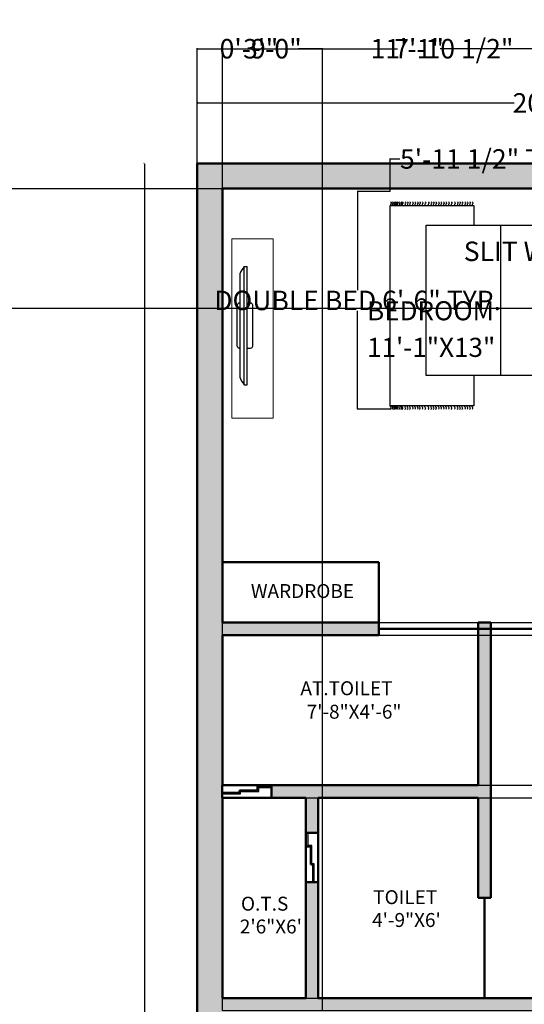
# Model space of a CAD drawing. Units: inches. Extents: x 48 to 822, y -191 to 651.
# Tile 11 of 13: x 445 to 626, y 297 to 651. Entities that reach past the tile are written whole.
import ezdxf

# ---------------------------------------------------------------- set-up
doc = ezdxf.new("R2010")
doc.units = ezdxf.units.IN
doc.header["$MEASUREMENT"] = 0
doc.layers.get('0').update_dxf_attribs({"color": 254})
for name, color, linetype, lineweight in [('A-ANNO-DIMS', 2, 'Continuous', 18), ('A-AREA-IDEN', 7, 'Continuous', 25), ('A-FURN', 8, 'Continuous', 18), ('A-GLAZ', 4, 'Continuous', 25), ('A-WALL', 7, 'Continuous', 50), ('A-WALL-PATT', 8, 'Continuous', 13)]:
    doc.layers.add(name, color=color, linetype=linetype, lineweight=lineweight)
doc.layers.add('furniture', color=250, linetype='Continuous')
doc.styles.get("Standard").update_dxf_attribs({"font": 'arial.ttf'})
doc.dimstyles.get("Standard").update_dxf_attribs({"dimtxt": 7, "dimasz": 0.18, "dimexe": 0.18, "dimexo": 0.0625, "dimgap": 0.09, "dimtad": 0, "dimtih": 1, "dimtoh": 1, "dimzin": 0, "dimdsep": 46, "dimlunit": 3, "dimtxsty": 'Standard', "dimcen": 0.09, "dimadec": 0, "dimazin": 0, "dimtfac": 1, "dimtofl": 0, "dimtmove": 0, "dimatfit": 3, "dimfxl": 1, "dimtolj": 1, "dimtzin": 0, "dimarcsym": 0})

# ---------------------------------------------------------------- blocks, each defined once
blk = doc.blocks.new('CARPET')
at = {"layer": 'furniture'}
for p, q in [((-51.53, -98.11), (-51.53, -55.12)), ((-51.53, -55.12), (-41.27, -55.12)), ((36, -55.12), (51.55, -55.12)), ((51.55, -55.12), (51.55, -98.11)), ((51.55, -98.11), (-51.53, -98.11))]:
    blk.add_line(p, q, dxfattribs=at)
for points, knots in [([(-53.37, -55.99), (-53.22, -55.8), (-52.9, -55.41), (-52.34, -55.8), (-51.89, -56.08), (-51.65, -55.91), (-51.53, -55.83)], [0, 0, 0, 0, 0.653278, 1.290138, 1.740457, 2.114451, 2.114451, 2.114451, 2.114451]), ([(53.37, -55.99), (53.22, -55.8), (52.9, -55.41), (52.34, -55.8), (51.89, -56.08), (51.65, -55.91), (51.53, -55.83)], [0, 0, 0, 0, 0.653278, 1.290138, 1.740457, 2.114451, 2.114451, 2.114451, 2.114451]), ([(-53.37, -57.26), (-53.22, -57.07), (-52.9, -56.67), (-52.34, -57.07), (-51.89, -57.35), (-51.65, -57.17), (-51.53, -57.1)], [0, 0, 0, 0, 0.653278, 1.290138, 1.740457, 2.114451, 2.114451, 2.114451, 2.114451]), ([(-53.37, -58.59), (-53.22, -58.4), (-52.9, -58.01), (-52.34, -58.4), (-51.89, -58.68), (-51.65, -58.5), (-51.53, -58.43)], [0, 0, 0, 0, 0.653278, 1.290138, 1.740457, 2.114451, 2.114451, 2.114451, 2.114451]), ([(-53.37, -59.78), (-53.22, -59.58), (-52.9, -59.19), (-52.34, -59.58), (-51.89, -59.86), (-51.65, -59.69), (-51.53, -59.61)], [0, 0, 0, 0, 0.653278, 1.290138, 1.740457, 2.114451, 2.114451, 2.114451, 2.114451]), ([(-53.37, -61.22), (-53.22, -61.02), (-52.9, -60.63), (-52.34, -61.02), (-51.89, -61.3), (-51.65, -61.13), (-51.53, -61.05)], [0, 0, 0, 0, 0.653278, 1.290138, 1.740457, 2.114451, 2.114451, 2.114451, 2.114451]), ([(53.37, -57.26), (53.22, -57.07), (52.9, -56.67), (52.34, -57.07), (51.89, -57.35), (51.65, -57.17), (51.53, -57.1)], [0, 0, 0, 0, 0.653278, 1.290138, 1.740457, 2.114451, 2.114451, 2.114451, 2.114451]), ([(53.37, -58.59), (53.22, -58.4), (52.9, -58.01), (52.34, -58.4), (51.89, -58.68), (51.65, -58.5), (51.53, -58.43)], [0, 0, 0, 0, 0.653278, 1.290138, 1.740457, 2.114451, 2.114451, 2.114451, 2.114451]), ([(53.37, -59.78), (53.22, -59.58), (52.9, -59.19), (52.34, -59.58), (51.89, -59.86), (51.65, -59.69), (51.53, -59.61)], [0, 0, 0, 0, 0.653278, 1.290138, 1.740457, 2.114451, 2.114451, 2.114451, 2.114451]), ([(53.37, -61.22), (53.22, -61.02), (52.9, -60.63), (52.34, -61.02), (51.89, -61.3), (51.65, -61.13), (51.53, -61.05)], [0, 0, 0, 0, 0.653278, 1.290138, 1.740457, 2.114451, 2.114451, 2.114451, 2.114451]), ([(-53.37, -62.44), (-53.22, -62.25), (-52.9, -61.86), (-52.34, -62.25), (-51.89, -62.53), (-51.65, -62.36), (-51.53, -62.28)], [0, 0, 0, 0, 0.653278, 1.290138, 1.740457, 2.114451, 2.114451, 2.114451, 2.114451]), ([(-53.37, -63.63), (-53.22, -63.43), (-52.9, -63.04), (-52.34, -63.43), (-51.89, -63.72), (-51.65, -63.54), (-51.53, -63.46)], [0, 0, 0, 0, 0.653278, 1.290138, 1.740457, 2.114451, 2.114451, 2.114451, 2.114451]), ([(-53.37, -65.07), (-53.22, -64.87), (-52.9, -64.48), (-52.34, -64.87), (-51.89, -65.15), (-51.65, -64.98), (-51.53, -64.9)], [0, 0, 0, 0, 0.653278, 1.290138, 1.740457, 2.114451, 2.114451, 2.114451, 2.114451]), ([(53.37, -62.44), (53.22, -62.25), (52.9, -61.86), (52.34, -62.25), (51.89, -62.53), (51.65, -62.36), (51.53, -62.28)], [0, 0, 0, 0, 0.653278, 1.290138, 1.740457, 2.114451, 2.114451, 2.114451, 2.114451]), ([(53.37, -63.63), (53.22, -63.43), (52.9, -63.04), (52.34, -63.43), (51.89, -63.72), (51.65, -63.54), (51.53, -63.46)], [0, 0, 0, 0, 0.653278, 1.290138, 1.740457, 2.114451, 2.114451, 2.114451, 2.114451]), ([(53.37, -65.07), (53.22, -64.87), (52.9, -64.48), (52.34, -64.87), (51.89, -65.15), (51.65, -64.98), (51.53, -64.9)], [0, 0, 0, 0, 0.653278, 1.290138, 1.740457, 2.114451, 2.114451, 2.114451, 2.114451]), ([(-53.37, -66.76), (-53.22, -66.56), (-52.9, -66.17), (-52.34, -66.56), (-51.89, -66.84), (-51.65, -66.67), (-51.53, -66.59)], [0, 0, 0, 0, 0.653278, 1.290138, 1.740457, 2.114451, 2.114451, 2.114451, 2.114451]), ([(-53.37, -68.2), (-53.22, -68), (-52.9, -67.61), (-52.34, -68), (-51.89, -68.28), (-51.65, -68.11), (-51.53, -68.03)], [0, 0, 0, 0, 0.653278, 1.290138, 1.740457, 2.114451, 2.114451, 2.114451, 2.114451]), ([(-53.37, -69.53), (-53.22, -69.33), (-52.9, -68.94), (-52.34, -69.33), (-51.89, -69.61), (-51.65, -69.44), (-51.53, -69.36)], [0, 0, 0, 0, 0.653278, 1.290138, 1.740457, 2.114451, 2.114451, 2.114451, 2.114451]), ([(-53.37, -70.79), (-53.22, -70.6), (-52.9, -70.21), (-52.34, -70.6), (-51.89, -70.88), (-51.65, -70.7), (-51.53, -70.63)], [0, 0, 0, 0, 0.653278, 1.290138, 1.740457, 2.114451, 2.114451, 2.114451, 2.114451]), ([(53.37, -66.76), (53.22, -66.56), (52.9, -66.17), (52.34, -66.56), (51.89, -66.84), (51.65, -66.67), (51.53, -66.59)], [0, 0, 0, 0, 0.653278, 1.290138, 1.740457, 2.114451, 2.114451, 2.114451, 2.114451]), ([(53.37, -68.2), (53.22, -68), (52.9, -67.61), (52.34, -68), (51.89, -68.28), (51.65, -68.11), (51.53, -68.03)], [0, 0, 0, 0, 0.653278, 1.290138, 1.740457, 2.114451, 2.114451, 2.114451, 2.114451]), ([(53.37, -69.53), (53.22, -69.33), (52.9, -68.94), (52.34, -69.33), (51.89, -69.61), (51.65, -69.44), (51.53, -69.36)], [0, 0, 0, 0, 0.653278, 1.290138, 1.740457, 2.114451, 2.114451, 2.114451, 2.114451]), ([(53.37, -70.79), (53.22, -70.6), (52.9, -70.21), (52.34, -70.6), (51.89, -70.88), (51.65, -70.7), (51.53, -70.63)], [0, 0, 0, 0, 0.653278, 1.290138, 1.740457, 2.114451, 2.114451, 2.114451, 2.114451]), ([(-53.37, -72.12), (-53.22, -71.93), (-52.9, -71.54), (-52.34, -71.93), (-51.89, -72.21), (-51.65, -72.04), (-51.53, -71.96)], [0, 0, 0, 0, 0.653278, 1.290138, 1.740457, 2.114451, 2.114451, 2.114451, 2.114451]), ([(-53.37, -73.31), (-53.22, -73.11), (-52.9, -72.72), (-52.34, -73.11), (-51.89, -73.4), (-51.65, -73.22), (-51.53, -73.14)], [0, 0, 0, 0, 0.653278, 1.290138, 1.740457, 2.114451, 2.114451, 2.114451, 2.114451]), ([(-53.37, -74.75), (-53.22, -74.55), (-52.9, -74.16), (-52.34, -74.55), (-51.89, -74.83), (-51.65, -74.66), (-51.53, -74.58)], [0, 0, 0, 0, 0.653278, 1.290138, 1.740457, 2.114451, 2.114451, 2.114451, 2.114451]), ([(-53.37, -75.98), (-53.22, -75.78), (-52.9, -75.39), (-52.34, -75.78), (-51.89, -76.06), (-51.65, -75.89), (-51.53, -75.81)], [0, 0, 0, 0, 0.653278, 1.290138, 1.740457, 2.114451, 2.114451, 2.114451, 2.114451]), ([(53.37, -72.12), (53.22, -71.93), (52.9, -71.54), (52.34, -71.93), (51.89, -72.21), (51.65, -72.04), (51.53, -71.96)], [0, 0, 0, 0, 0.653278, 1.290138, 1.740457, 2.114451, 2.114451, 2.114451, 2.114451]), ([(53.37, -73.31), (53.22, -73.11), (52.9, -72.72), (52.34, -73.11), (51.89, -73.4), (51.65, -73.22), (51.53, -73.14)], [0, 0, 0, 0, 0.653278, 1.290138, 1.740457, 2.114451, 2.114451, 2.114451, 2.114451]), ([(53.37, -74.75), (53.22, -74.55), (52.9, -74.16), (52.34, -74.55), (51.89, -74.83), (51.65, -74.66), (51.53, -74.58)], [0, 0, 0, 0, 0.653278, 1.290138, 1.740457, 2.114451, 2.114451, 2.114451, 2.114451]), ([(53.37, -75.98), (53.22, -75.78), (52.9, -75.39), (52.34, -75.78), (51.89, -76.06), (51.65, -75.89), (51.53, -75.81)], [0, 0, 0, 0, 0.653278, 1.290138, 1.740457, 2.114451, 2.114451, 2.114451, 2.114451]), ([(-53.37, -77.16), (-53.22, -76.96), (-52.9, -76.57), (-52.34, -76.96), (-51.89, -77.25), (-51.65, -77.07), (-51.53, -76.99)], [0, 0, 0, 0, 0.653278, 1.290138, 1.740457, 2.114451, 2.114451, 2.114451, 2.114451]), ([(-53.37, -78.6), (-53.22, -78.4), (-52.9, -78.01), (-52.34, -78.4), (-51.89, -78.68), (-51.65, -78.51), (-51.53, -78.43)], [0, 0, 0, 0, 0.653278, 1.290138, 1.740457, 2.114451, 2.114451, 2.114451, 2.114451]), ([(-53.37, -80.29), (-53.22, -80.09), (-52.9, -79.7), (-52.34, -80.09), (-51.89, -80.37), (-51.65, -80.2), (-51.53, -80.12)], [0, 0, 0, 0, 0.653278, 1.290138, 1.740457, 2.114451, 2.114451, 2.114451, 2.114451]), ([(53.37, -77.16), (53.22, -76.96), (52.9, -76.57), (52.34, -76.96), (51.89, -77.25), (51.65, -77.07), (51.53, -76.99)], [0, 0, 0, 0, 0.653278, 1.290138, 1.740457, 2.114451, 2.114451, 2.114451, 2.114451]), ([(53.37, -78.6), (53.22, -78.4), (52.9, -78.01), (52.34, -78.4), (51.89, -78.68), (51.65, -78.51), (51.53, -78.43)], [0, 0, 0, 0, 0.653278, 1.290138, 1.740457, 2.114451, 2.114451, 2.114451, 2.114451]), ([(53.37, -80.29), (53.22, -80.09), (52.9, -79.7), (52.34, -80.09), (51.89, -80.37), (51.65, -80.2), (51.53, -80.12)], [0, 0, 0, 0, 0.653278, 1.290138, 1.740457, 2.114451, 2.114451, 2.114451, 2.114451]), ([(-53.37, -81.73), (-53.22, -81.53), (-52.9, -81.14), (-52.34, -81.53), (-51.89, -81.81), (-51.65, -81.64), (-51.53, -81.56)], [0, 0, 0, 0, 0.653278, 1.290138, 1.740457, 2.114451, 2.114451, 2.114451, 2.114451]), ([(-53.37, -83.06), (-53.22, -82.86), (-52.9, -82.47), (-52.34, -82.86), (-51.89, -83.14), (-51.65, -82.97), (-51.53, -82.89)], [0, 0, 0, 0, 0.653278, 1.290138, 1.740457, 2.114451, 2.114451, 2.114451, 2.114451]), ([(-53.37, -84.18), (-53.22, -83.99), (-52.9, -83.6), (-52.34, -83.99), (-51.89, -84.27), (-51.65, -84.09), (-51.53, -84.02)], [0, 0, 0, 0, 0.653278, 1.290138, 1.740457, 2.114451, 2.114451, 2.114451, 2.114451]), ([(-53.37, -85.51), (-53.22, -85.32), (-52.9, -84.93), (-52.34, -85.32), (-51.89, -85.6), (-51.65, -85.42), (-51.53, -85.35)], [0, 0, 0, 0, 0.653278, 1.290138, 1.740457, 2.114451, 2.114451, 2.114451, 2.114451]), ([(53.37, -81.73), (53.22, -81.53), (52.9, -81.14), (52.34, -81.53), (51.89, -81.81), (51.65, -81.64), (51.53, -81.56)], [0, 0, 0, 0, 0.653278, 1.290138, 1.740457, 2.114451, 2.114451, 2.114451, 2.114451]), ([(53.37, -83.06), (53.22, -82.86), (52.9, -82.47), (52.34, -82.86), (51.89, -83.14), (51.65, -82.97), (51.53, -82.89)], [0, 0, 0, 0, 0.653278, 1.290138, 1.740457, 2.114451, 2.114451, 2.114451, 2.114451]), ([(53.37, -84.18), (53.22, -83.99), (52.9, -83.6), (52.34, -83.99), (51.89, -84.27), (51.65, -84.09), (51.53, -84.02)], [0, 0, 0, 0, 0.653278, 1.290138, 1.740457, 2.114451, 2.114451, 2.114451, 2.114451]), ([(53.37, -85.51), (53.22, -85.32), (52.9, -84.93), (52.34, -85.32), (51.89, -85.6), (51.65, -85.42), (51.53, -85.35)], [0, 0, 0, 0, 0.653278, 1.290138, 1.740457, 2.114451, 2.114451, 2.114451, 2.114451]), ([(-53.37, -86.7), (-53.22, -86.5), (-52.9, -86.11), (-52.34, -86.5), (-51.89, -86.78), (-51.65, -86.61), (-51.53, -86.53)], [0, 0, 0, 0, 0.653278, 1.290138, 1.740457, 2.114451, 2.114451, 2.114451, 2.114451]), ([(-53.37, -88.14), (-53.22, -87.94), (-52.9, -87.55), (-52.34, -87.94), (-51.89, -88.22), (-51.65, -88.05), (-51.53, -87.97)], [0, 0, 0, 0, 0.653278, 1.290138, 1.740457, 2.114451, 2.114451, 2.114451, 2.114451]), ([(-53.37, -89.36), (-53.22, -89.17), (-52.9, -88.78), (-52.34, -89.17), (-51.89, -89.45), (-51.65, -89.28), (-51.53, -89.2)], [0, 0, 0, 0, 0.653278, 1.290138, 1.740457, 2.114451, 2.114451, 2.114451, 2.114451]), ([(-53.37, -90.55), (-53.22, -90.35), (-52.9, -89.96), (-52.34, -90.35), (-51.89, -90.64), (-51.65, -90.46), (-51.53, -90.38)], [0, 0, 0, 0, 0.653278, 1.290138, 1.740457, 2.114451, 2.114451, 2.114451, 2.114451]), ([(53.37, -86.7), (53.22, -86.5), (52.9, -86.11), (52.34, -86.5), (51.89, -86.78), (51.65, -86.61), (51.53, -86.53)], [0, 0, 0, 0, 0.653278, 1.290138, 1.740457, 2.114451, 2.114451, 2.114451, 2.114451]), ([(53.37, -88.14), (53.22, -87.94), (52.9, -87.55), (52.34, -87.94), (51.89, -88.22), (51.65, -88.05), (51.53, -87.97)], [0, 0, 0, 0, 0.653278, 1.290138, 1.740457, 2.114451, 2.114451, 2.114451, 2.114451]), ([(53.37, -89.36), (53.22, -89.17), (52.9, -88.78), (52.34, -89.17), (51.89, -89.45), (51.65, -89.28), (51.53, -89.2)], [0, 0, 0, 0, 0.653278, 1.290138, 1.740457, 2.114451, 2.114451, 2.114451, 2.114451]), ([(53.37, -90.55), (53.22, -90.35), (52.9, -89.96), (52.34, -90.35), (51.9, -90.63), (51.66, -90.47), (51.55, -90.4)], [0, 0, 0, 0, 0.653278, 1.290138, 1.740457, 2.0926, 2.0926, 2.0926, 2.0926]), ([(-53.37, -91.99), (-53.22, -91.79), (-52.9, -91.4), (-52.34, -91.79), (-51.89, -92.07), (-51.65, -91.9), (-51.53, -91.82)], [0, 0, 0, 0, 0.653278, 1.290138, 1.740457, 2.114451, 2.114451, 2.114451, 2.114451]), ([(-53.37, -92.69), (-53.22, -92.48), (-52.9, -92.08), (-52.35, -92.49), (-51.89, -92.77), (-51.65, -92.6), (-51.53, -92.52)], [0, 0, 0, 0, 0.663904, 1.307406, 1.757725, 2.131719, 2.131719, 2.131719, 2.131719]), ([(-53.37, -93.61), (-53.22, -93.42), (-52.9, -93.03), (-52.34, -93.42), (-51.89, -93.7), (-51.65, -93.52), (-51.53, -93.45)], [0, 0, 0, 0, 0.653278, 1.290138, 1.740457, 2.114451, 2.114451, 2.114451, 2.114451]), ([(-53.37, -94.55), (-53.22, -94.35), (-52.9, -93.96), (-52.34, -94.35), (-51.89, -94.63), (-51.65, -94.46), (-51.53, -94.38)], [0, 0, 0, 0, 0.653278, 1.290138, 1.740457, 2.114451, 2.114451, 2.114451, 2.114451]), ([(-53.37, -95.05), (-53.22, -94.85), (-52.9, -94.46), (-52.34, -94.85), (-51.89, -95.14), (-51.65, -94.96), (-51.53, -94.88)], [0, 0, 0, 0, 0.653278, 1.290138, 1.740457, 2.114451, 2.114451, 2.114451, 2.114451]), ([(-53.37, -95.73), (-53.22, -95.54), (-52.9, -95.15), (-52.34, -95.54), (-51.89, -95.82), (-51.65, -95.65), (-51.53, -95.57)], [0, 0, 0, 0, 0.653278, 1.290138, 1.740457, 2.114451, 2.114451, 2.114451, 2.114451]), ([(-53.37, -96.38), (-53.22, -96.18), (-52.9, -95.79), (-52.34, -96.18), (-51.89, -96.47), (-51.65, -96.29), (-51.53, -96.21)], [0, 0, 0, 0, 0.653278, 1.290138, 1.740457, 2.114451, 2.114451, 2.114451, 2.114451]), ([(53.37, -95.78), (53.22, -95.58), (52.9, -95.19), (52.34, -95.58), (51.89, -95.86), (51.65, -95.69), (51.53, -95.61)], [0, 0, 0, 0, 0.653278, 1.290138, 1.740457, 2.114451, 2.114451, 2.114451, 2.114451]), ([(53.37, -96.43), (53.22, -96.23), (52.9, -95.84), (52.34, -96.23), (51.89, -96.51), (51.65, -96.34), (51.53, -96.26)], [0, 0, 0, 0, 0.653278, 1.290138, 1.740457, 2.114451, 2.114451, 2.114451, 2.114451]), ([(53.37, -91.99), (53.22, -91.79), (52.9, -91.4), (52.34, -91.79), (51.9, -92.07), (51.66, -91.91), (51.55, -91.83)], [0, 0, 0, 0, 0.653278, 1.290138, 1.740457, 2.0926, 2.0926, 2.0926, 2.0926]), ([(53.37, -92.69), (53.22, -92.49), (52.9, -92.09), (52.34, -92.49), (51.9, -92.77), (51.66, -92.61), (51.55, -92.53)], [0, 0, 0, 0, 0.656792, 1.295826, 1.746145, 2.098292, 2.098292, 2.098292, 2.098292]), ([(53.37, -93.66), (53.22, -93.46), (52.9, -93.07), (52.34, -93.46), (51.9, -93.74), (51.66, -93.58), (51.55, -93.5)], [0, 0, 0, 0, 0.653278, 1.290138, 1.740457, 2.0926, 2.0926, 2.0926, 2.0926]), ([(53.37, -94.59), (53.22, -94.4), (52.9, -94.01), (52.34, -94.4), (51.9, -94.68), (51.66, -94.51), (51.55, -94.44)], [0, 0, 0, 0, 0.653278, 1.290138, 1.740457, 2.0926, 2.0926, 2.0926, 2.0926]), ([(53.37, -95.1), (53.22, -94.9), (52.9, -94.51), (52.34, -94.9), (51.9, -95.18), (51.66, -95.02), (51.55, -94.94)], [0, 0, 0, 0, 0.653278, 1.290138, 1.740457, 2.0926, 2.0926, 2.0926, 2.0926]), ([(-53.37, -97.17), (-53.22, -96.98), (-52.9, -96.59), (-52.34, -96.98), (-51.89, -97.26), (-51.65, -97.08), (-51.53, -97.01)], [0, 0, 0, 0, 0.653278, 1.290138, 1.740457, 2.114451, 2.114451, 2.114451, 2.114451]), ([(-53.37, -97.99), (-53.22, -97.79), (-52.9, -97.4), (-52.34, -97.79), (-51.89, -98.08), (-51.65, -97.9), (-51.53, -97.82)], [0, 0, 0, 0, 0.653278, 1.290138, 1.740457, 2.114451, 2.114451, 2.114451, 2.114451]), ([(53.37, -97.22), (53.22, -97.02), (52.9, -96.63), (52.34, -97.02), (51.89, -97.3), (51.65, -97.13), (51.53, -97.05)], [0, 0, 0, 0, 0.653278, 1.290138, 1.740457, 2.114451, 2.114451, 2.114451, 2.114451]), ([(53.37, -97.99), (53.22, -97.79), (52.9, -97.4), (52.34, -97.79), (51.89, -98.08), (51.65, -97.9), (51.53, -97.82)], [0, 0, 0, 0, 0.653278, 1.290138, 1.740457, 2.114451, 2.114451, 2.114451, 2.114451])]:
    blk.add_open_spline(points, degree=3, knots=knots, dxfattribs=at)
blk = doc.blocks.new('A$C58D270C6')
at = {"layer": 'furniture'}
for p, q in [((9.09, 124.13), (9.09, 108.87)), ((1.46, 116.5), (16.73, 116.5)), ((14.97, 94.84), (24.62, 107.92)), ((24.62, 94.93), (24.62, 107.92)), ((42.08, 108), (42.08, 36)), ((14.97, 94.93), (24.62, 94.93)), ((14.97, 94.84), (14.97, 36)), ((16.22, 94.93), (16.22, 36)), ((9.25, 36), (9.25, 20.74)), ((1.62, 28.37), (16.88, 28.37))]:
    blk.add_line(p, q, dxfattribs=at)
for points in [[(18.5, 108), (18.34, 124.13), (-0.16, 124.13), (0, 108)], [(0, 108), (77.91, 108), (77.91, 36), (0, 36)], [(4.09, 94.93), (14.97, 94.93), (14.97, 73.83), (4.09, 73.83)], [(4.09, 65.23), (14.97, 65.23), (14.97, 44.13), (4.09, 44.13)], [(18.65, 19.87), (18.5, 36), (0, 36), (0.16, 19.87)]]:
    blk.add_lwpolyline(points, close=True, dxfattribs=at)
for centre in [(9.09, 116.5), (9.25, 28.37)]:
    blk.add_circle(centre, 5.95, dxfattribs=at)
at = {"layer": 'furniture', "xscale": 0.9312884925094044, "yscale": 0.9312884925094044, "zscale": 0.9312884925094044, "rotation": 90}
blk.add_blockref('CARPET', (3.79, 74.47), dxfattribs=at)
blk = doc.blocks.new('PLASMA-LARGE')
at = {"layer": 'furniture'}
for p, q in [((-7.26, 0), (7.26, 0)), ((-21, -2.5), (21, -2.5)), ((-21, -2.5), (-21, -3.5)), ((-18.61, -1), (18.61, -1)), ((-8, -1), (-8, -0.74)), ((8, -1), (8, -0.74)), ((21, -2.5), (21, -3.5)), ((-21, -3.5), (21, -3.5)), ((-8, -3.5), (-8, -4.76)), ((-7.26, -5.5), (7.26, -5.5)), ((8, -3.5), (8, -4.76))]:
    blk.add_line(p, q, dxfattribs=at)
for centre, radius, start, end in [((-7.26, -0.74), 0.744, 90, 180), ((7.26, -0.74), 0.744, 0, 90), ((-13.97, -11.05), 11.07, 114.7602, 129.4175), ((13.97, -11.05), 11.07, 50.5825, 65.2398), ((-7.26, -4.76), 0.744, 180, 270), ((7.26, -4.76), 0.744, 270, 0)]:
    blk.add_arc(centre, radius, start, end, dxfattribs=at)
blk = doc.blocks.new('*D18')
at = {"layer": 'A-ANNO-DIMS', "color": 0, "lineweight": -2, "transparency": 16777216}
for p, q in [((508.61, 621.85), (508.61, 621.28)), ((508.79, 621.46), (622.52, 621.46)), ((748.43, 621.46), (634.7, 621.46)), ((748.61, 621.85), (748.61, 621.28))]:
    blk.add_line(p, q, dxfattribs=at)
at = {"layer": 'A-ANNO-DIMS', "color": 0, "transparency": 16777216}
for points in [[(508.79, 621.49), (508.79, 621.43), (508.61, 621.46)], [(748.43, 621.49), (748.43, 621.43), (748.61, 621.46)]]:
    blk.add_solid(points, dxfattribs=at)
at = {"layer": 'Defpoints', "color": 0, "transparency": 16777216}
for p in [(508.61, 621.91), (748.61, 621.91), (748.61, 621.46)]:
    blk.add_point(p, dxfattribs=at)
at = {"layer": 'A-ANNO-DIMS', "color": 0, "transparency": 16777216, "insert": (628.61, 621.46), "char_height": 7, "attachment_point": 5}
blk.add_mtext("\\A1;20'", dxfattribs=at)
blk = doc.blocks.new('*D19')
at = {"layer": 'A-ANNO-DIMS', "color": 0, "lineweight": -2, "transparency": 16777216}
for p, q in [((489.56, 599.69), (489.41, 599.69)), ((489.59, 599.51), (489.59, 243.35)), ((489.59, -120.13), (489.59, 236.02)), ((489.56, -120.31), (489.41, -120.31))]:
    blk.add_line(p, q, dxfattribs=at)
at = {"layer": 'A-ANNO-DIMS', "color": 0, "transparency": 16777216}
for points in [[(489.56, 599.51), (489.62, 599.51), (489.59, 599.69)], [(489.56, -120.13), (489.62, -120.13), (489.59, -120.31)]]:
    blk.add_solid(points, dxfattribs=at)
at = {"layer": 'Defpoints', "color": 0, "transparency": 16777216}
for p in [(489.62, 599.69), (489.59, -120.31), (489.62, -120.31)]:
    blk.add_point(p, dxfattribs=at)
at = {"layer": 'A-ANNO-DIMS', "color": 0, "transparency": 16777216, "insert": (489.59, 239.69), "char_height": 7, "attachment_point": 5}
blk.add_mtext("\\A1;60'", dxfattribs=at)
blk = doc.blocks.new('WIN-450')
for p, q in [((152.3, 373.99), (152.3, 375.35)), ((152.3, 375.35), (156.91, 375.35)), ((139.16, 373.13), (145.74, 373.13)), ((145.74, 373.13), (145.74, 373.99)), ((145.74, 373.99), (152.3, 373.99))]:
    blk.add_line(p, q)
blk = doc.blocks.new('TV-UNIT')
for p, q in [((14.9, 64.44), (0, 64.44)), ((0, 64.44), (0, 0)), ((14.9, 64.44), (14.9, 0)), ((0, 0), (14.9, 0))]:
    blk.add_line(p, q)
blk = doc.blocks.new('*D40')
at = {"layer": 'A-ANNO-DIMS', "color": 0, "lineweight": -2, "transparency": 16777216}
for p, q in [((577.94, 589.57), (566.08, 589.57)), ((566.26, 589.39), (566.26, 554.17)), ((566.26, 511.52), (566.26, 546.74)), ((577.94, 511.34), (566.08, 511.34))]:
    blk.add_line(p, q, dxfattribs=at)
at = {"layer": 'A-ANNO-DIMS', "color": 0, "transparency": 16777216}
for points in [[(566.23, 589.39), (566.29, 589.39), (566.26, 589.57)], [(566.23, 511.52), (566.29, 511.52), (566.26, 511.34)]]:
    blk.add_solid(points, dxfattribs=at)
at = {"layer": 'Defpoints', "color": 0, "transparency": 16777216}
for p in [(578, 589.57), (566.26, 511.34), (578, 511.34)]:
    blk.add_point(p, dxfattribs=at)
at = {"layer": 'A-ANNO-DIMS', "color": 0, "transparency": 16777216, "insert": (566.26, 550.46), "char_height": 7, "attachment_point": 5}
blk.add_mtext('\\A1;DOUBLE BED 6\'-6" TYP.', dxfattribs=at)
blk = doc.blocks.new('*D41')
at = {"layer": 'A-ANNO-DIMS', "color": 0, "lineweight": -2, "transparency": 16777216}
for p, q in [((578, 589.63), (578, 601.49)), ((578.18, 601.31), (581.44, 601.31)), ((649.3, 601.31), (646.04, 601.31)), ((649.48, 589.63), (649.48, 601.49))]:
    blk.add_line(p, q, dxfattribs=at)
at = {"layer": 'A-ANNO-DIMS', "color": 0, "transparency": 16777216}
for points in [[(578.18, 601.34), (578.18, 601.28), (578, 601.31)], [(649.3, 601.34), (649.3, 601.28), (649.48, 601.31)]]:
    blk.add_solid(points, dxfattribs=at)
at = {"layer": 'Defpoints', "color": 0, "transparency": 16777216}
for p in [(578, 601.31), (578, 589.57), (649.48, 589.57)]:
    blk.add_point(p, dxfattribs=at)
at = {"layer": 'A-ANNO-DIMS', "color": 0, "transparency": 16777216, "insert": (613.74, 601.31), "char_height": 7, "attachment_point": 5}
blk.add_mtext('\\A1;5\'-11 1/2" TYP.', dxfattribs=at)
blk = doc.blocks.new('*D50')
at = {"layer": 'A-ANNO-DIMS', "color": 0, "lineweight": -2, "transparency": 16777216}
for p, q in [((655.17, 585.52), (660.51, 585.52)), ((660.33, 585.34), (660.33, 571.83)), ((660.33, 550.9), (660.33, 564.41)), ((655.17, 550.72), (660.51, 550.72))]:
    blk.add_line(p, q, dxfattribs=at)
at = {"layer": 'A-ANNO-DIMS', "color": 0, "transparency": 16777216}
for points in [[(660.3, 585.34), (660.36, 585.34), (660.33, 585.52)], [(660.3, 550.9), (660.36, 550.9), (660.33, 550.72)]]:
    blk.add_solid(points, dxfattribs=at)
at = {"layer": 'Defpoints', "color": 0, "transparency": 16777216}
for p in [(655.11, 585.52), (660.33, 585.52), (655.11, 550.72)]:
    blk.add_point(p, dxfattribs=at)
at = {"layer": 'A-ANNO-DIMS', "color": 0, "transparency": 16777216, "insert": (660.33, 568.12), "char_height": 7, "attachment_point": 5}
blk.add_mtext('\\A1;SLIT WINDOW 2\'-11" TYP.', dxfattribs=at)
blk = doc.blocks.new('*D84')
at = {"layer": 'A-ANNO-DIMS', "color": 0, "lineweight": -2, "transparency": 16777216}
for p, q in [((356.51, 590.69), (790.04, 590.69)), ((789.86, 590.51), (789.86, 572.87)), ((789.86, 547.91), (789.86, 565.54)), ((356.51, 547.73), (790.04, 547.73))]:
    blk.add_line(p, q, dxfattribs=at)
at = {"layer": 'A-ANNO-DIMS', "color": 0, "transparency": 16777216}
for points in [[(789.83, 590.51), (789.89, 590.51), (789.86, 590.69)], [(789.83, 547.91), (789.89, 547.91), (789.86, 547.73)]]:
    blk.add_solid(points, dxfattribs=at)
at = {"layer": 'Defpoints', "color": 0, "transparency": 16777216}
for p in [(356.45, 590.69), (356.45, 547.73), (789.86, 547.73)]:
    blk.add_point(p, dxfattribs=at)
at = {"layer": 'A-ANNO-DIMS', "color": 0, "transparency": 16777216, "insert": (789.86, 569.21), "char_height": 7, "attachment_point": 5}
blk.add_mtext('\\A1;3\'-7"', dxfattribs=at)
blk = doc.blocks.new('*D96')
at = {"layer": 'A-ANNO-DIMS', "color": 0, "lineweight": -2, "transparency": 16777216}
for p, q in [((508.61, 599.75), (508.61, 641.12)), ((508.79, 640.94), (517.43, 640.94)), ((517.61, 590.75), (517.61, 641.12)), ((517.61, 640.94), (517.79, 640.94))]:
    blk.add_line(p, q, dxfattribs=at)
at = {"layer": 'A-ANNO-DIMS', "color": 0, "transparency": 16777216}
for points in [[(508.79, 640.97), (508.79, 640.91), (508.61, 640.94)], [(517.43, 640.97), (517.43, 640.91), (517.61, 640.94)]]:
    blk.add_solid(points, dxfattribs=at)
at = {"layer": 'Defpoints', "color": 0, "transparency": 16777216}
for p in [(517.61, 640.94), (508.61, 599.69), (517.61, 590.69)]:
    blk.add_point(p, dxfattribs=at)
at = {"layer": 'A-ANNO-DIMS', "color": 0, "transparency": 16777216, "insert": (527.18, 640.94), "char_height": 7, "attachment_point": 5}
blk.add_mtext('\\A1;0\'-9"', dxfattribs=at)
blk = doc.blocks.new('*D97')
at = {"layer": 'A-ANNO-DIMS', "color": 0, "lineweight": -2, "transparency": 16777216}
for p, q in [((517.61, 590.75), (517.61, 641.12)), ((517.79, 640.94), (572.33, 640.94)), ((650.43, 640.94), (595.89, 640.94)), ((650.61, 590.75), (650.61, 641.12))]:
    blk.add_line(p, q, dxfattribs=at)
at = {"layer": 'A-ANNO-DIMS', "color": 0, "transparency": 16777216}
for points in [[(517.79, 640.97), (517.79, 640.91), (517.61, 640.94)], [(650.43, 640.97), (650.43, 640.91), (650.61, 640.94)]]:
    blk.add_solid(points, dxfattribs=at)
at = {"layer": 'Defpoints', "color": 0, "transparency": 16777216}
for p in [(650.61, 640.94), (517.61, 590.69), (650.61, 590.69)]:
    blk.add_point(p, dxfattribs=at)
at = {"layer": 'A-ANNO-DIMS', "color": 0, "transparency": 16777216, "insert": (584.11, 640.94), "char_height": 7, "attachment_point": 5}
blk.add_mtext('\\A1;11\'-1"', dxfattribs=at)
blk = doc.blocks.new('*D105')
at = {"layer": 'A-ANNO-DIMS', "color": 0, "lineweight": -2, "transparency": 16777216}
for p, q in [((517.67, 590.69), (790.04, 590.69)), ((789.86, 590.51), (789.86, 516.35)), ((789.86, 434.87), (789.86, 509.02)), ((517.67, 434.69), (790.04, 434.69))]:
    blk.add_line(p, q, dxfattribs=at)
at = {"layer": 'A-ANNO-DIMS', "color": 0, "transparency": 16777216}
for points in [[(789.83, 590.51), (789.89, 590.51), (789.86, 590.69)], [(789.83, 434.87), (789.89, 434.87), (789.86, 434.69)]]:
    blk.add_solid(points, dxfattribs=at)
at = {"layer": 'Defpoints', "color": 0, "transparency": 16777216}
for p in [(517.61, 590.69), (517.61, 434.69), (789.86, 434.69)]:
    blk.add_point(p, dxfattribs=at)
at = {"layer": 'A-ANNO-DIMS', "color": 0, "transparency": 16777216, "insert": (789.86, 512.69), "char_height": 7, "attachment_point": 5}
blk.add_mtext('\\A1;13\'-0"', dxfattribs=at)
blk = doc.blocks.new('*D106')
at = {"layer": 'A-ANNO-DIMS', "color": 0, "lineweight": -2, "transparency": 16777216}
for p, q in [((517.67, 434.69), (790.04, 434.69)), ((789.86, 434.51), (789.86, 430.37)), ((517.67, 430.19), (790.04, 430.19)), ((789.86, 430.01), (789.68, 430.01)), ((789.86, 430.19), (789.86, 430.01))]:
    blk.add_line(p, q, dxfattribs=at)
at = {"layer": 'A-ANNO-DIMS', "color": 0, "transparency": 16777216}
for points in [[(789.83, 434.51), (789.89, 434.51), (789.86, 434.69)], [(789.83, 430.37), (789.89, 430.37), (789.86, 430.19)]]:
    blk.add_solid(points, dxfattribs=at)
at = {"layer": 'Defpoints', "color": 0, "transparency": 16777216}
for p in [(517.61, 434.69), (517.61, 430.19), (789.86, 430.19)]:
    blk.add_point(p, dxfattribs=at)
at = {"layer": 'A-ANNO-DIMS', "color": 0, "transparency": 16777216, "insert": (772.13, 430.01), "char_height": 7, "attachment_point": 5}
blk.add_mtext('\\A1;0\'-4 1/2"', dxfattribs=at)
blk = doc.blocks.new('*D107')
at = {"layer": 'A-ANNO-DIMS', "color": 0, "lineweight": -2, "transparency": 16777216}
for p, q in [((517.67, 430.19), (790.04, 430.19)), ((789.86, 430.01), (789.86, 406.85)), ((789.86, 376.37), (789.86, 399.52)), ((517.67, 376.19), (790.04, 376.19))]:
    blk.add_line(p, q, dxfattribs=at)
at = {"layer": 'A-ANNO-DIMS', "color": 0, "transparency": 16777216}
for points in [[(789.83, 430.01), (789.89, 430.01), (789.86, 430.19)], [(789.83, 376.37), (789.89, 376.37), (789.86, 376.19)]]:
    blk.add_solid(points, dxfattribs=at)
at = {"layer": 'Defpoints', "color": 0, "transparency": 16777216}
for p in [(517.61, 430.19), (517.61, 376.19), (789.86, 376.19)]:
    blk.add_point(p, dxfattribs=at)
at = {"layer": 'A-ANNO-DIMS', "color": 0, "transparency": 16777216, "insert": (789.86, 403.19), "char_height": 7, "attachment_point": 5}
blk.add_mtext('\\A1;4\'-6"', dxfattribs=at)
blk = doc.blocks.new('*D108')
at = {"layer": 'A-ANNO-DIMS', "color": 0, "lineweight": -2, "transparency": 16777216}
for p, q in [((517.67, 376.19), (790.04, 376.19)), ((789.86, 376.01), (789.86, 371.87)), ((517.67, 371.69), (790.04, 371.69)), ((789.86, 371.69), (789.86, 371.51)), ((789.86, 371.51), (789.68, 371.51))]:
    blk.add_line(p, q, dxfattribs=at)
at = {"layer": 'A-ANNO-DIMS', "color": 0, "transparency": 16777216}
for points in [[(789.83, 376.01), (789.89, 376.01), (789.86, 376.19)], [(789.83, 371.87), (789.89, 371.87), (789.86, 371.69)]]:
    blk.add_solid(points, dxfattribs=at)
at = {"layer": 'Defpoints', "color": 0, "transparency": 16777216}
for p in [(517.61, 376.19), (517.61, 371.69), (789.86, 371.69)]:
    blk.add_point(p, dxfattribs=at)
at = {"layer": 'A-ANNO-DIMS', "color": 0, "transparency": 16777216, "insert": (772.13, 371.51), "char_height": 7, "attachment_point": 5}
blk.add_mtext('\\A1;0\'-4 1/2"', dxfattribs=at)
blk = doc.blocks.new('*D109')
at = {"layer": 'A-ANNO-DIMS', "color": 0, "lineweight": -2, "transparency": 16777216}
for p, q in [((517.67, 371.69), (790.04, 371.69)), ((789.86, 371.51), (789.86, 339.35)), ((789.86, 299.87), (789.86, 332.02)), ((517.67, 299.69), (790.04, 299.69))]:
    blk.add_line(p, q, dxfattribs=at)
at = {"layer": 'A-ANNO-DIMS', "color": 0, "transparency": 16777216}
for points in [[(789.83, 371.51), (789.89, 371.51), (789.86, 371.69)], [(789.83, 299.87), (789.89, 299.87), (789.86, 299.69)]]:
    blk.add_solid(points, dxfattribs=at)
at = {"layer": 'Defpoints', "color": 0, "transparency": 16777216}
for p in [(517.61, 371.69), (517.61, 299.69), (789.86, 299.69)]:
    blk.add_point(p, dxfattribs=at)
at = {"layer": 'A-ANNO-DIMS', "color": 0, "transparency": 16777216, "insert": (789.86, 335.69), "char_height": 7, "attachment_point": 5}
blk.add_mtext('\\A1;6\'-0"', dxfattribs=at)
blk = doc.blocks.new('*D110')
at = {"layer": 'A-ANNO-DIMS', "color": 0, "lineweight": -2, "transparency": 16777216}
for p, q in [((517.67, 299.69), (790.04, 299.69)), ((789.86, 299.51), (789.86, 295.37)), ((517.67, 295.19), (790.04, 295.19)), ((789.86, 295.01), (789.68, 295.01)), ((789.86, 295.19), (789.86, 295.01))]:
    blk.add_line(p, q, dxfattribs=at)
at = {"layer": 'A-ANNO-DIMS', "color": 0, "transparency": 16777216}
for points in [[(789.83, 299.51), (789.89, 299.51), (789.86, 299.69)], [(789.83, 295.37), (789.89, 295.37), (789.86, 295.19)]]:
    blk.add_solid(points, dxfattribs=at)
at = {"layer": 'Defpoints', "color": 0, "transparency": 16777216}
for p in [(517.61, 299.69), (517.61, 295.19), (789.86, 295.19)]:
    blk.add_point(p, dxfattribs=at)
at = {"layer": 'A-ANNO-DIMS', "color": 0, "transparency": 16777216, "insert": (772.13, 295.01), "char_height": 7, "attachment_point": 5}
blk.add_mtext('\\A1;0\'-4 1/2"', dxfattribs=at)
blk = doc.blocks.new('*D124')
at = {"layer": 'A-ANNO-DIMS', "color": 0, "lineweight": -2, "transparency": 16777216}
for p, q in [((517.61, 295.25), (517.61, 641.12)), ((517.79, 640.94), (526.22, 640.94)), ((553.43, 640.94), (545, 640.94)), ((553.61, 295.25), (553.61, 641.12))]:
    blk.add_line(p, q, dxfattribs=at)
at = {"layer": 'A-ANNO-DIMS', "color": 0, "transparency": 16777216}
for points in [[(517.79, 640.97), (517.79, 640.91), (517.61, 640.94)], [(553.43, 640.97), (553.43, 640.91), (553.61, 640.94)]]:
    blk.add_solid(points, dxfattribs=at)
at = {"layer": 'Defpoints', "color": 0, "transparency": 16777216}
for p in [(553.61, 640.94), (517.61, 295.19), (553.61, 295.19)]:
    blk.add_point(p, dxfattribs=at)
at = {"layer": 'A-ANNO-DIMS', "color": 0, "transparency": 16777216, "insert": (535.61, 640.94), "char_height": 7, "attachment_point": 5}
blk.add_mtext('\\A1;3\'-0"', dxfattribs=at)
blk = doc.blocks.new('*D126')
at = {"layer": 'A-ANNO-DIMS', "color": 0, "lineweight": -2, "transparency": 16777216}
for p, q in [((553.61, 295.25), (553.61, 641.12)), ((553.79, 640.94), (580.61, 640.94)), ((647.91, 640.94), (621.09, 640.94)), ((648.09, 295.25), (648.09, 641.12))]:
    blk.add_line(p, q, dxfattribs=at)
at = {"layer": 'A-ANNO-DIMS', "color": 0, "transparency": 16777216}
for points in [[(553.79, 640.97), (553.79, 640.91), (553.61, 640.94)], [(647.91, 640.97), (647.91, 640.91), (648.09, 640.94)]]:
    blk.add_solid(points, dxfattribs=at)
at = {"layer": 'Defpoints', "color": 0, "transparency": 16777216}
for p in [(648.09, 640.94), (553.61, 295.19), (648.09, 295.19)]:
    blk.add_point(p, dxfattribs=at)
at = {"layer": 'A-ANNO-DIMS', "color": 0, "transparency": 16777216, "insert": (600.85, 640.94), "char_height": 7, "attachment_point": 5}
blk.add_mtext('\\A1;7\'-10 1/2"', dxfattribs=at)

msp = doc.modelspace()

# ---------------------------------------------------------------- hatches: boundary and pattern name
at = {"layer": 'A-GLAZ'}
h = msp.add_hatch(color=256, dxfattribs=at)
h.dxf.hatch_style = 1
h.paths.add_polyline_path([(524.113, 373.987), (530.673, 373.987), (530.673, 375.346), (535.284, 375.346), (535.284, 375.689), (530.292, 375.689), (530.292, 374.347), (523.809, 374.347), (523.809, 373.472), (517.534, 373.472), (517.534, 373.126), (524.113, 373.126)])
h = msp.add_hatch(color=256, dxfattribs=at)
h.dxf.hatch_style = 1
h.paths.add_polyline_path([(549.81, 347.948), (549.81, 354.509), (548.451, 354.509), (548.451, 359.12), (548.108, 359.12), (548.108, 354.128), (549.45, 354.128), (549.45, 347.645), (550.325, 347.645), (550.325, 341.37), (550.671, 341.37), (550.671, 347.948)])
at = {"layer": 'A-WALL-PATT'}
h = msp.add_hatch(color=256, dxfattribs=at)
h.dxf.hatch_style = 1
h.paths.add_polyline_path([(614.11, 432.437), (609.61, 432.437), (609.61, 376.187), (535.284, 376.187), (535.284, 371.687), (547.61, 371.687), (547.61, 359.12), (552.11, 359.12), (552.11, 371.687), (609.61, 371.687), (609.61, 335.687), (614.11, 335.687)], flags=17)
h.paths.add_polyline_path([(614.11, 434.687), (609.61, 434.687), (609.61, 432.437), (614.11, 432.437)], flags=17)
h.paths.add_polyline_path([(573.934, 434.687), (517.61, 434.687), (517.61, 590.687), (650.61, 590.687), (650.61, 585.522), (655.11, 585.522), (655.11, 590.687), (739.61, 590.687), (739.61, 548.687), (655.11, 548.687), (655.11, 550.72), (650.61, 550.72), (650.61, 458.608), (655.11, 458.608), (655.11, 544.187), (739.61, 544.187), (739.61, 434.541), (650.61, 434.541), (650.61, 430.041), (739.61, 430.041), (739.61, -16.844), (729.973, -16.844), (729.973, -21.344), (748.61, -21.344), (748.61, 599.687), (508.61, 599.687), (508.61, -120.313), (543.114, -120.313), (543.114, -111.313), (517.61, -111.313), (517.61, 38.687), (607.29, 38.687), (607.29, 43.187), (517.61, 43.187), (517.61, 97.187), (654.61, 97.187), (654.61, 30.562), (659.11, 30.562), (659.11, 101.895), (654.61, 101.895), (654.61, 101.687), (517.61, 101.687), (517.61, 221.687), (654.61, 221.687), (654.61, 218.066), (659.11, 218.066), (659.11, 226.187), (517.61, 226.187), (517.61, 295.187), (614.11, 295.187), (648.087, 295.187), (661.07, 295.187), (661.07, 299.687), (614.11, 299.687), (552.11, 299.687), (552.11, 341.37), (547.61, 341.37), (547.61, 299.687), (517.61, 299.687), (517.61, 371.687), (517.534, 371.687), (517.534, 376.187), (517.61, 430.187), (573.934, 430.187)])
h.paths.add_polyline_path([(659.11, -87.328), (654.61, -87.328), (654.61, -111.313), (598.94, -111.313), (598.94, -120.313), (659.11, -120.313)], flags=0)
h.paths.add_polyline_path([(671.266, -16.844), (659.11, -16.844), (659.11, -12.05), (654.61, -12.05), (654.61, -31.502), (659.11, -31.502), (659.11, -21.344), (671.266, -21.344)], flags=17)
h.paths.add_polyline_path([(606.11, 97.187), (601.61, 97.187), (601.61, 75.902), (606.11, 75.902)], flags=17)
h.paths.add_polyline_path([(659.11, 169.875), (654.61, 169.875), (654.61, 157.721), (659.11, 157.721)], flags=17)

# ---------------------------------------------------------------- linework, layer by layer
at = {"layer": 'A-WALL'}
for p, q in [((508.61, 599.687), (748.61, 599.687)), ((508.61, -120.313), (508.61, 599.687)), ((517.61, 590.687), (650.61, 590.687)), ((517.61, 434.687), (517.61, 590.687)), ((573.934, 456.373), (517.61, 456.373)), ((573.934, 434.687), (573.934, 456.373)), ((517.61, 434.687), (573.934, 434.687)), ((573.934, 434.687), (573.934, 430.187)), ((573.934, 432.437), (614.11, 432.437)), ((609.61, 434.687), (614.11, 434.687)), ((609.61, 376.187), (609.61, 434.687)), ((614.11, 335.687), (614.11, 434.687)), ((614.11, 432.437), (650.61, 432.437)), ((517.61, 430.187), (573.934, 430.187)), ((517.61, 376.187), (517.61, 430.187)), ((517.534, 376.187), (517.534, 371.687)), ((535.284, 376.187), (517.534, 376.187)), ((517.61, 376.187), (609.61, 376.187)), ((530.292, 374.347), (530.292, 375.689)), ((530.292, 375.689), (535.284, 375.689)), ((535.284, 371.687), (535.284, 376.187)), ((517.534, 373.472), (523.809, 373.472)), ((517.534, 371.687), (535.284, 371.687)), ((517.61, 371.687), (547.61, 371.687)), ((517.61, 299.687), (517.61, 371.687)), ((523.809, 373.472), (523.809, 374.347)), ((523.809, 374.347), (530.292, 374.347)), ((547.61, 299.687), (547.61, 371.687)), ((552.11, 371.687), (609.61, 371.687)), ((552.11, 299.687), (552.11, 371.687)), ((609.61, 335.687), (609.61, 371.687)), ((552.11, 359.12), (547.61, 359.12)), ((547.61, 359.12), (547.61, 341.37)), ((552.11, 341.37), (552.11, 359.12)), ((549.45, 354.128), (548.108, 354.128)), ((549.45, 347.645), (549.45, 354.128)), ((550.325, 347.645), (549.45, 347.645)), ((550.325, 341.37), (550.325, 347.645)), ((547.61, 341.37), (552.11, 341.37)), ((609.61, 335.687), (614.11, 335.687)), ((611.86, 335.687), (611.86, 299.687)), ((517.61, 299.687), (547.61, 299.687)), ((552.11, 299.687), (614.11, 299.687)), ((614.11, 299.687), (661.07, 299.687))]:
    msp.add_line(p, q, dxfattribs=at)

# ---------------------------------------------------------------- block references
at = {"layer": 'A-FURN'}
for name, p, xscale, yscale, zscale, rotation in [('A$C58D270C6', (649.367, 604.474), 0.7500000390647866, 0.7500000390647866, 0.7500000390647866, 180), ('PLASMA-LARGE', (522.968, 541.397), 1.011294184530666, 1.011294184530666, 1.011294184530666, 90.00000000000003)]:
    msp.add_blockref(name, p, dxfattribs=dict(at, xscale=xscale, yscale=yscale, zscale=zscale, rotation=rotation))
msp.add_blockref('TV-UNIT', (521.018, 508.136), dxfattribs=at)
at = {"layer": 'A-GLAZ'}
msp.add_blockref('WIN-450', (378.375, 0), dxfattribs=at)
at = {"layer": 'A-GLAZ', "rotation": 90.01545447568515}
msp.add_blockref('WIN-450', (923.838, 202.312), dxfattribs=at)

# ---------------------------------------------------------------- texts
at = {"layer": 'A-AREA-IDEN'}
for s, height, p in [('BEDROOM', 6.866, (569.664, 543.314)), ('11\'-1"X13"', 6.866, (569.664, 530.155)), ('WARDROBE', 5.0075, (527.863, 443.488)), ('AT.TOILET', 5.0075, (545.68, 408.546)), ('7\'-8"X4\'-6"', 5.00749, (547.919, 400.108)), ('TOILET', 5.0075, (571.867, 333.442)), ('O.T.S', 5.0075, (524.309, 331.103)), ('4\'-9"X6\'', 5.0075, (571.463, 325.238)), ('2\'6"X6\'', 5.0075, (523.905, 322.9))]:
    msp.add_text(s, height=height, dxfattribs=at).set_placement(p)

# ---------------------------------------------------------------- dimensions: what is measured, and where the dimension line sits
at = {"layer": 'A-ANNO-DIMS'}
for base, p1, p2, override, picture, middle in [((648.087, 640.937), (553.61, 295.187), (648.087, 295.187), {"dimdec": 1, "dimlfac": 1, "dimrnd": 0, "dimzin": 1, "dimdsep": 46, "dimlunit": 4, "dimfrac": 2}, '*D126', (600.849, 640.937)), ((517.61, 640.937), (508.61, 599.687), (517.61, 590.687), {"dimdec": 1, "dimlfac": 1, "dimrnd": 0, "dimzin": 1, "dimdsep": 46, "dimlunit": 4, "dimfrac": 2}, '*D96', (527.184, 640.937)), ((650.61, 640.937), (517.61, 590.687), (650.61, 590.687), {"dimdec": 1, "dimlfac": 1, "dimrnd": 0, "dimzin": 1, "dimdsep": 46, "dimlunit": 4, "dimfrac": 2}, '*D97', (584.11, 640.937)), ((553.61, 640.937), (517.61, 295.187), (553.61, 295.187), {"dimdec": 1, "dimlfac": 1, "dimrnd": 0, "dimzin": 1, "dimdsep": 46, "dimlunit": 4, "dimfrac": 2}, '*D124', (535.61, 640.937)), ((748.61, 621.465), (508.61, 621.913), (748.61, 621.913), {"dimclrd": 0, "dimclre": 0, "dimclrt": 0}, '*D18', (628.61, 621.465))]:
    dim = msp.add_linear_dim(base=base, p1=p1, p2=p2, dimstyle='Standard', override=override, dxfattribs=at)
    dim.commit()
    dim.dimension.update_dxf_attribs({"geometry": picture, "text_midpoint": middle})
for base, p1, p2, angle, text, picture, middle in [((577.998, 601.307), (649.484, 589.572), (577.998, 589.572), 180, '<> TYP.', '*D41', (613.741, 601.307)), ((566.263, 511.339), (577.998, 589.572), (577.998, 511.339), 270, 'DOUBLE BED <> TYP.', '*D40', (566.263, 550.455)), ((660.331, 585.522), (655.11, 550.72), (655.11, 585.522), 90, 'SLIT WINDOW <> TYP.', '*D50', (660.331, 568.121))]:
    dim = msp.add_linear_dim(base=base, p1=p1, p2=p2, angle=angle, text=text, dimstyle='Standard', override={"dimdec": 1, "dimlfac": 1, "dimrnd": 0, "dimzin": 1, "dimdsep": 46, "dimlunit": 4, "dimfrac": 2}, dxfattribs=at)
    dim.commit()
    dim.dimension.update_dxf_attribs({"geometry": picture, "text_midpoint": middle})
for base, p1, p2, override, picture, middle in [((489.59, -120.313), (489.619, 599.687), (489.619, -120.313), {"dimclrd": 0, "dimclre": 0, "dimclrt": 0}, '*D19', (489.59, 239.687)), ((789.86, 547.726), (356.451, 590.687), (356.451, 547.726), {"dimdec": 1, "dimlfac": 1, "dimrnd": 0, "dimzin": 1, "dimdsep": 46, "dimlunit": 4, "dimfrac": 2}, '*D84', (789.86, 569.206)), ((789.86, 434.687), (517.61, 590.687), (517.61, 434.687), {"dimdec": 1, "dimlfac": 1, "dimrnd": 0, "dimzin": 1, "dimdsep": 46, "dimlunit": 4, "dimfrac": 2}, '*D105', (789.86, 512.687)), ((789.86, 430.187), (517.61, 434.687), (517.61, 430.187), {"dimdec": 1, "dimlfac": 1, "dimrnd": 0, "dimzin": 1, "dimdsep": 46, "dimlunit": 4, "dimfrac": 2}, '*D106', (772.131, 430.007)), ((789.86, 376.187), (517.61, 430.187), (517.61, 376.187), {"dimdec": 1, "dimlfac": 1, "dimrnd": 0, "dimzin": 1, "dimdsep": 46, "dimlunit": 4, "dimfrac": 2}, '*D107', (789.86, 403.187)), ((789.86, 371.687), (517.61, 376.187), (517.61, 371.687), {"dimdec": 1, "dimlfac": 1, "dimrnd": 0, "dimzin": 1, "dimdsep": 46, "dimlunit": 4, "dimfrac": 2}, '*D108', (772.131, 371.507)), ((789.86, 299.687), (517.61, 371.687), (517.61, 299.687), {"dimdec": 1, "dimlfac": 1, "dimrnd": 0, "dimzin": 1, "dimdsep": 46, "dimlunit": 4, "dimfrac": 2}, '*D109', (789.86, 335.687)), ((789.86, 295.187), (517.61, 299.687), (517.61, 295.187), {"dimdec": 1, "dimlfac": 1, "dimrnd": 0, "dimzin": 1, "dimdsep": 46, "dimlunit": 4, "dimfrac": 2}, '*D110', (772.131, 295.007))]:
    dim = msp.add_linear_dim(base=base, p1=p1, p2=p2, angle=90, dimstyle='Standard', override=override, dxfattribs=at)
    dim.commit()
    dim.dimension.update_dxf_attribs({"geometry": picture, "text_midpoint": middle})

doc.saveas('drawing.dxf')
